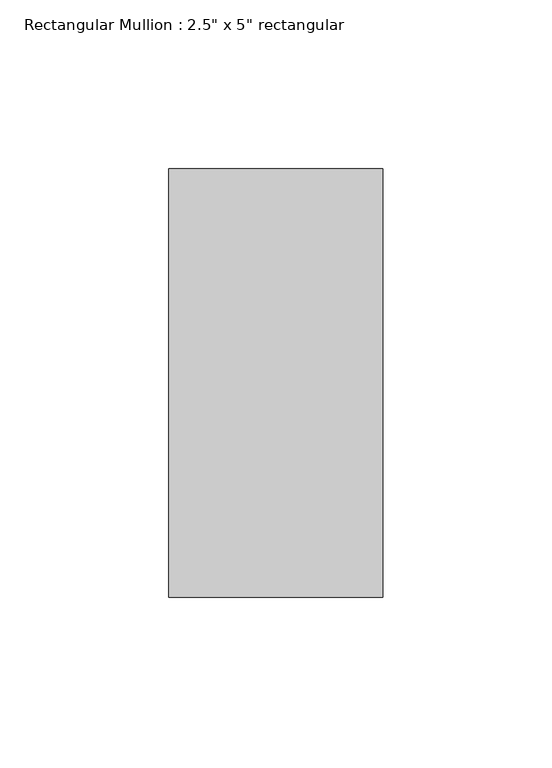
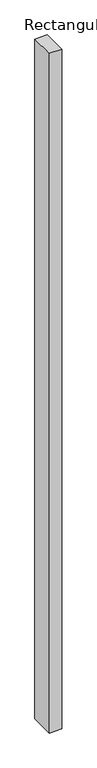
"""IFC4 building model written with IfcOpenShell, lengths in millimetres: member geometry."""

from ifc_helpers import new_model, si_unit, frame, origin, place, context, project, spatial, polyline, outline, extrude, source, transform, mapped, element, save


def member_4d31274b(model_context):
    return source(origin(), model_context, "Body", "SweptSolid", [
        extrude(outline(polyline([(0.0, 63.5), (0.0, -63.5), (-63.5, -63.5), (-63.5, 63.5), (0.0, 63.5)])), frame((0.0, 0.0, -3657.6), z_axis=(0.0, 0.0, 1.0), x_axis=(1.0, 0.0, 0.0)), (0.0, 0.0, 1.0), 3657.6),
    ])


if __name__ == "__main__":
    model = new_model("IFC4")
    model_context = context("Model", 3, world=origin())
    ifc_project = project(units=[si_unit("LENGTHUNIT", "METRE", prefix="MILLI")], contexts=[model_context])
    site = spatial("IfcSite", under=ifc_project)
    building = spatial("IfcBuilding", under=site)
    placement = place(None, origin())
    member_shape = member_4d31274b(model_context)
    element("IfcMember", 1, ObjectType="Rectangular Mullion : 2.5\" x 5\" rectangular", at=placement, inside=building, context=model_context, shape_type="MappedRepresentation", body=[
        mapped(member_shape, transform((0.0, 0.0, 0.0), x_axis=(1.0, 0.0, 0.0), y_axis=(0.0, 1.0, 0.0), z_axis=(0.0, 0.0, 1.0))),
    ])
    save(model, "model.ifc")

# Revit data of these elements
# Type "Rectangular Mullion : 2.5\" x 5\" rectangular"
#   built-in parameter 1007304 = 0.416667 (stored number, unit not read)
#   built-in parameter 1007301 = 0.104167 (stored number, unit not read)
#   built-in parameter 1007300 = 0.104167 (stored number, unit not read)
# Element 1 (IfcMember, "Rectangular Mullion : 2.5\" x 5\" rectangular")
#   Materials on its faces: "Iron, Ductile"
# Materials
#   "Iron, Ductile": class "Metal", colour RGB 0 0 0, transparency 0, Description = "Ductile cast iron", Cost = 0
